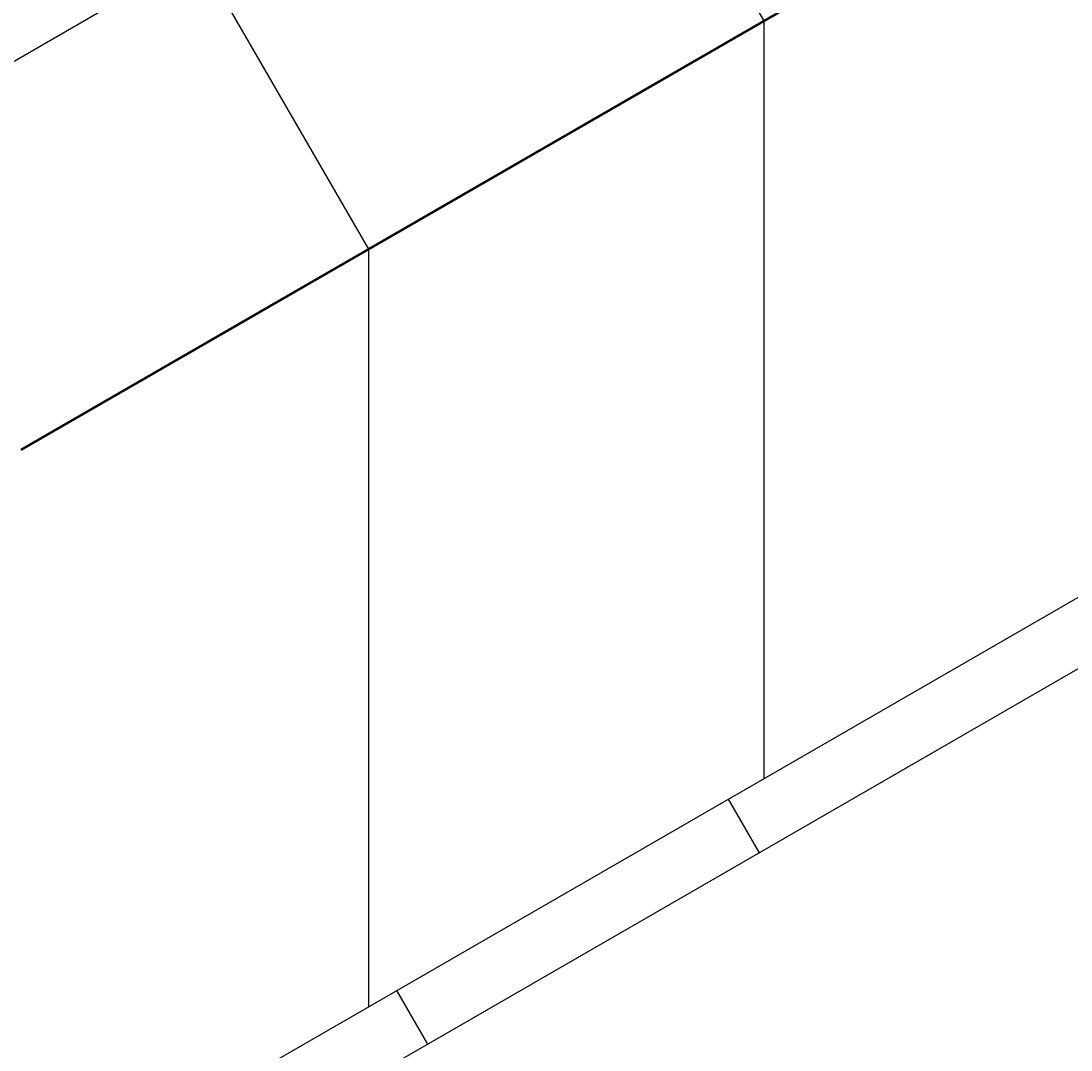
# Model space of a CAD drawing. Units: metres. Extents: x -2391 to 4922, y -635 to 4845.
# Tile 20 of 37: x -1008 to 31, y 3011 to 4030. Entities that reach past the tile are written whole.
import ezdxf

# ---------------------------------------------------------------- set-up
doc = ezdxf.new("R2010")
doc.units = ezdxf.units.M
doc.header["$MEASUREMENT"] = 0
for name, color, linetype, lineweight in [('A-ANNO-DIMS', 2, 'Continuous', 18), ('A-FLOR-FIXT', 3, 'Continuous', 25), ('A-WALL', 7, 'Continuous', 50)]:
    doc.layers.add(name, color=color, linetype=linetype, lineweight=lineweight)
doc.styles.get("Standard").update_dxf_attribs({"font": 'arial.ttf'})
doc.dimstyles.get("Standard").update_dxf_attribs({"dimtxt": 5, "dimasz": 4, "dimexe": 0.18, "dimexo": 0.0625, "dimgap": 0.09, "dimtad": 0, "dimtih": 1, "dimtoh": 1, "dimdec": 0, "dimzin": 0, "dimdsep": 46, "dimtxsty": 'Standard', "dimcen": 0.09, "dimadec": 0, "dimazin": 0, "dimtfac": 1, "dimtdec": 0, "dimtofl": 0, "dimtmove": 0, "dimatfit": 3, "dimfxl": 1, "dimtolj": 1, "dimtzin": 0, "dimarcsym": 0})

# ---------------------------------------------------------------- blocks, each defined once
blk = doc.blocks.new('*D9')
at = {"layer": 'A-ANNO-DIMS', "color": 0, "lineweight": -2, "transparency": 16777216}
for p, q in [((-2047.3, 3005.3), (-2047.3, 4842)), ((-2043.3, 4841.8), (-755.9, 4841.8)), ((546.7, 4841.8), (-740.7, 4841.8)), ((550.7, 4505.3), (550.7, 4842))]:
    blk.add_line(p, q, dxfattribs=at)
at = {"layer": 'A-ANNO-DIMS', "color": 0, "transparency": 16777216}
for points in [[(-2043.3, 4842.4), (-2043.3, 4841.1), (-2047.3, 4841.8)], [(546.7, 4842.4), (546.7, 4841.1), (550.7, 4841.8)]]:
    blk.add_solid(points, dxfattribs=at)
at = {"layer": 'Defpoints', "color": 0, "transparency": 16777216}
for p in [(550.7, 4841.8), (550.7, 4505.3), (-2047.3, 3005.3)]:
    blk.add_point(p, dxfattribs=at)
at = {"layer": 'A-ANNO-DIMS', "color": 0, "transparency": 16777216, "insert": (-748.3, 4841.8), "char_height": 5, "attachment_point": 5}
blk.add_mtext('\\A1;2598', dxfattribs=at)
blk = doc.blocks.new('*D10')
at = {"layer": 'A-ANNO-DIMS', "color": 0, "lineweight": -2, "transparency": 16777216}
for p, q in [((550.7, 4505.3), (-2384, 4505.3)), ((-2383.8, 4501.3), (-2383.8, 2107.9)), ((-2383.8, -290.7), (-2383.8, 2102.6)), ((-488.6, -294.7), (-2384, -294.7))]:
    blk.add_line(p, q, dxfattribs=at)
at = {"layer": 'A-ANNO-DIMS', "color": 0, "transparency": 16777216}
for points in [[(-2384.5, 4501.3), (-2383.2, 4501.3), (-2383.8, 4505.3)], [(-2384.5, -290.7), (-2383.2, -290.7), (-2383.8, -294.7)]]:
    blk.add_solid(points, dxfattribs=at)
at = {"layer": 'Defpoints', "color": 0, "transparency": 16777216}
for p in [(-2383.8, 4505.3), (550.7, 4505.3), (-488.5, -294.7)]:
    blk.add_point(p, dxfattribs=at)
at = {"layer": 'A-ANNO-DIMS', "color": 0, "transparency": 16777216, "insert": (-2383.8, 2105.3), "char_height": 5, "attachment_point": 5}
blk.add_mtext('\\A1;4800', dxfattribs=at)
blk = doc.blocks.new('*D37')
at = {"layer": 'A-ANNO-DIMS', "color": 0, "lineweight": -2, "transparency": 16777216}
for p, q in [((-664, 3804), (-832.3, 4095.5)), ((-835.7, 4093.4), (-1050.8, 3969.2)), ((-1275.1, 3839.7), (-1060, 3963.9)), ((-1110.4, 3546.3), (-1278.7, 3837.8))]:
    blk.add_line(p, q, dxfattribs=at)
at = {"layer": 'A-ANNO-DIMS', "color": 0, "transparency": 16777216}
for points in [[(-836, 4094), (-835.4, 4092.8), (-832.2, 4095.4)], [(-1275.5, 3840.2), (-1274.8, 3839.1), (-1278.6, 3837.7)]]:
    blk.add_solid(points, dxfattribs=at)
at = {"layer": 'Defpoints', "color": 0, "transparency": 16777216}
for p in [(-832.2, 4095.4), (-664, 3804), (-1110.4, 3546.2)]:
    blk.add_point(p, dxfattribs=at)
at = {"layer": 'A-ANNO-DIMS', "color": 0, "transparency": 16777216, "insert": (-1055.4, 3966.5), "char_height": 5, "attachment_point": 5}
blk.add_mtext('\\A1;515.4', dxfattribs=at)
blk = doc.blocks.new('*D38')
at = {"layer": 'A-ANNO-DIMS', "color": 0, "lineweight": -2, "transparency": 16777216}
for p, q in [((-444.4, 4319.3), (-632, 4211)), ((-272.7, 4029.9), (-441, 4321.4)), ((-828.8, 4097.4), (-641.2, 4205.7)), ((-664, 3804), (-832.3, 4095.5))]:
    blk.add_line(p, q, dxfattribs=at)
at = {"layer": 'A-ANNO-DIMS', "color": 0, "transparency": 16777216}
for points in [[(-444.8, 4319.9), (-444.1, 4318.7), (-441, 4321.3)], [(-829.1, 4098), (-828.4, 4096.8), (-832.2, 4095.4)]]:
    blk.add_solid(points, dxfattribs=at)
at = {"layer": 'Defpoints', "color": 0, "transparency": 16777216}
for p in [(-441, 4321.3), (-272.7, 4029.9), (-664, 3804)]:
    blk.add_point(p, dxfattribs=at)
at = {"layer": 'A-ANNO-DIMS', "color": 0, "transparency": 16777216, "insert": (-636.6, 4208.3), "char_height": 5, "attachment_point": 5}
blk.add_mtext('\\A1;451.8', dxfattribs=at)
blk = doc.blocks.new('*D41')
at = {"layer": 'A-ANNO-DIMS', "color": 0, "lineweight": -2, "transparency": 16777216}
for p, q in [((-2047.3, 3005.3), (-1879, 3296.8)), ((-1875.6, 3294.7), (-1104.2, 2849.3)), ((-323.7, 2398.7), (-1095.1, 2844.1)), ((-488.5, 2105.3), (-320.1, 2396.8))]:
    blk.add_line(p, q, dxfattribs=at)
at = {"layer": 'A-ANNO-DIMS', "color": 0, "transparency": 16777216}
for points in [[(-1875.3, 3295.3), (-1876, 3294.1), (-1879.1, 3296.7)], [(-323.4, 2399.3), (-324, 2398.1), (-320.2, 2396.7)]]:
    blk.add_solid(points, dxfattribs=at)
at = {"layer": 'Defpoints', "color": 0, "transparency": 16777216}
for p in [(-2047.3, 3005.3), (-320.2, 2396.7), (-488.5, 2105.3)]:
    blk.add_point(p, dxfattribs=at)
at = {"layer": 'A-ANNO-DIMS', "color": 0, "transparency": 16777216, "insert": (-1099.7, 2846.7), "char_height": 5, "attachment_point": 5}
blk.add_mtext('\\A1;1800', dxfattribs=at)

msp = doc.modelspace()

# ---------------------------------------------------------------- linework, layer by layer
at = {"layer": 'A-FLOR-FIXT'}
for p, q in [((-272.7053, 3279.8588), (-272.7053, 4029.8588)), ((-663.9742, 3053.9596), (-663.9742, 3803.9596)), ((612.0233, 3790.6571), (-878.2, 2930.2763)), ((612.0233, 3719.8954), (-816.9186, 2894.8954)), ((-308.1091, 3259.4184), (-277.4683, 3206.3472)), ((-605.5716, 3016.9166), (-636.2123, 3069.9879))]:
    msp.add_line(p, q, dxfattribs=at)
at = {"layer": 'A-WALL'}
msp.add_line((-1008.1038, 3605.2763), (550.7419, 4505.2763), dxfattribs=at)

# ---------------------------------------------------------------- dimensions: what is measured, and where the dimension line sits
at = {"layer": 'A-ANNO-DIMS'}
dim = msp.add_linear_dim(base=(550.7419, 4841.7763), p1=(-2047.3343, 3005.2763), p2=(550.7419, 4505.2763), dimstyle='Standard', override={"dimdec": 0, "dimlfac": 1, "dimrnd": 0, "dimzin": 0, "dimdsep": 46, "dimlunit": 2}, dxfattribs=at)
dim.commit()
dim.dimension.update_dxf_attribs({"geometry": '*D9', "text_midpoint": (-748.2962, 4841.7763)})
for base, p1, p2, angle, override, picture, middle in [((-2383.8343, 4505.2763), (-488.4886, -294.7237), (550.7419, 4505.2763), 90, {"dimdec": 0, "dimlfac": 1, "dimrnd": 0, "dimzin": 0, "dimdsep": 46, "dimlunit": 2}, '*D10', (-2383.8343, 2105.2763)), ((-440.9553, 4321.2764), (-663.9742, 3803.9596), (-272.7053, 4029.8588), 30, {"dimdec": 1, "dimlfac": 1, "dimrnd": 0, "dimzin": 0, "dimdsep": 46, "dimlunit": 2}, '*D38', (-636.5898, 4208.3267)), ((-832.2242, 4095.3771), (-1110.3549, 3546.2416), (-663.9742, 3803.9596), 30, {"dimdec": 1, "dimlfac": 1, "dimrnd": 0, "dimzin": 0, "dimdsep": 46, "dimlunit": 2}, '*D37', (-1055.4146, 3966.5181)), ((-320.2386, 2396.6938), (-2047.3343, 3005.2763), (-488.4886, 2105.2763), 330, {"dimdec": 0, "dimlfac": 1, "dimrnd": 0, "dimzin": 0, "dimdsep": 46, "dimlunit": 2}, '*D41', (-1099.6615, 2846.6938))]:
    dim = msp.add_linear_dim(base=base, p1=p1, p2=p2, angle=angle, dimstyle='Standard', override=override, dxfattribs=at)
    dim.commit()
    dim.dimension.update_dxf_attribs({"geometry": picture, "text_midpoint": middle})

doc.saveas('drawing.dxf')
